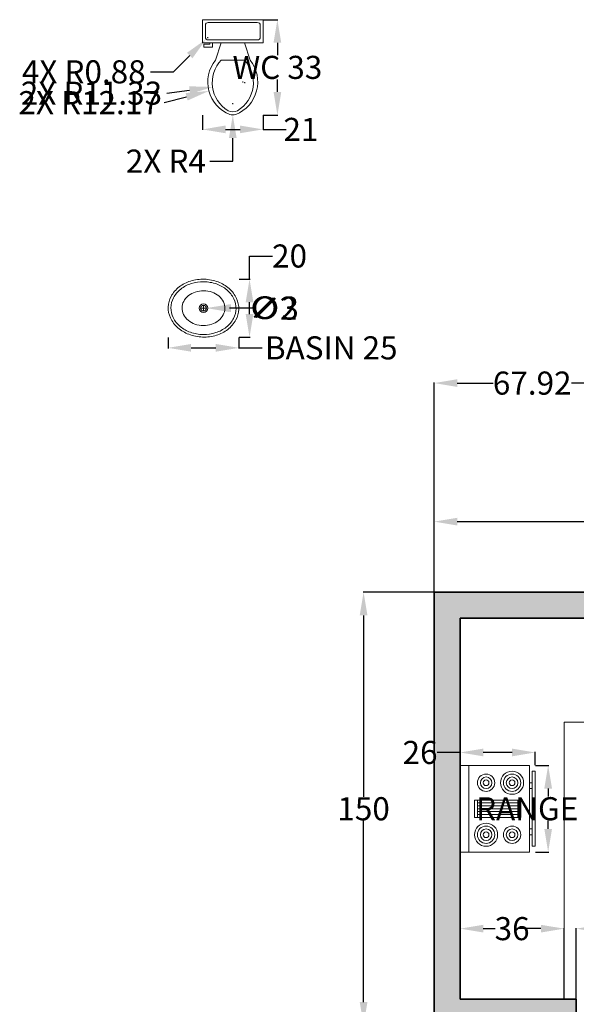
# Model space of a CAD drawing. Units: inches. Extents: x -52 to 678, y 23 to 685.
# Tile 6 of 11: x -52 to 141, y 334 to 675. Entities that reach past the tile are written whole.
import ezdxf

# ---------------------------------------------------------------- set-up
doc = ezdxf.new("R2010")
doc.units = ezdxf.units.IN
doc.header["$MEASUREMENT"] = 0
for name, color, linetype, lineweight in [('A-ANNO-DIMS', 2, 'Continuous', 18), ('A-EQPM', 8, 'Continuous', 18), ('A-FLOR-CASE', 8, 'Continuous', 18), ('A-FLOR-FIXT', 9, 'Continuous', 18), ('A-WALL', 7, 'Continuous', 35)]:
    doc.layers.add(name, color=color, linetype=linetype, lineweight=lineweight)
doc.layers.add('A-WALL-PATT', color=18, linetype='Continuous', lineweight=13, true_color=0x000000)
doc.styles.get("Standard").update_dxf_attribs({"font": 'arial.ttf'})
doc.dimstyles.get("Standard").update_dxf_attribs({"dimtxt": 8, "dimasz": 8, "dimexe": 0.18, "dimexo": 0.0625, "dimgap": 0.09, "dimtad": 0, "dimtih": 1, "dimtoh": 1, "dimdec": 0, "dimzin": 0, "dimdsep": 46, "dimlunit": 3, "dimtxsty": 'Standard', "dimcen": 0.09, "dimadec": 0, "dimazin": 0, "dimtfac": 1, "dimtdec": 0, "dimtofl": 0, "dimtmove": 0, "dimatfit": 3, "dimfxl": 1, "dimtolj": 1, "dimtzin": 0, "dimarcsym": 0})

# ---------------------------------------------------------------- blocks, each defined once
blk = doc.blocks.new('Range-Oven - 30 in top')
for p, q in [((0, -3), (30, -3)), ((12, -6), (18, -6)), ((13, -20), (13, -6)), ((14, -6), (14, -20)), ((15, -20), (15, -6)), ((16, -6), (16, -20)), ((17, -20), (17, -6)), ((18, -20), (12, -20)), ((6, -24), (6, -25)), ((8, -25), (8, -24)), ((22, -25), (22, -24)), ((24, -24), (24, -25))]:
    blk.add_line(p, q)
for points in [[(0, -24), (0, 0), (30, 0), (30, -24)], [(12, -21), (12, -5), (18, -5), (18, -21)], [(2, -26), (2, -25), (28, -25), (28, -26)]]:
    blk.add_lwpolyline(points, close=True)
for centre, radius in [((6, -9), 4), ((6, -9), 3), ((24, -9), 3), ((6, -9), 2), ((6, -9), 1), ((24, -9), 2), ((24, -9), 1), ((6, -18), 3), ((6, -18), 2), ((6, -18), 1), ((24, -18), 4), ((24, -18), 3), ((24, -18), 2), ((24, -18), 1)]:
    blk.add_circle(centre, radius)
blk = doc.blocks.new('Toilet - top')
for p, q in [((9.5, -6), (9.5, -2)), ((-10, -8.5), (-8, -8.5)), ((-10, -9.5), (-10, -8.5)), ((-7, -9.5), (-10, -9.5)), ((-8, -8.5), (-8, -8)), ((-7, -8), (-7, -9.5)), ((-4, -8), (-6, -14)), ((4, -8), (6, -14)), ((4, -14), (-4, -14))]:
    blk.add_line(p, q)
blk.add_lwpolyline([(10.5, -8), (10.5, 0), (-10.5, 0), (-10.5, -8)], close=True)
for points in [[(-9.5, -2), (-9.5, -6)], [(8.5, -1), (-8.5, -1)], [(-8.5, -7), (8.5, -7)]]:
    blk.add_lwpolyline(points)
for centre, radius, start, end in [((-8.62, -1.88), 0.884, 81.8699, 188.1301), ((8.62, -1.88), 0.884, 351.8699, 98.1301), ((-8.62, -6.12), 0.884, 171.8699, 278.1301), ((8.62, -6.12), 0.884, 261.8699, 8.1301), ((3.52, -21.58), 12.17, 141.4691, 247.9714), ((4.2, -21.82), 11.33, 136.3677, 238.9468), ((-3.52, -21.58), 12.17, 292.0284, 38.5307), ((-4.2, -21.82), 11.33, 301.053, 43.6321), ((0, -27.88), 4, 245.7318, 294.2682), ((0, -29), 4, 254.8605, 285.1395)]:
    blk.add_arc(centre, radius, start, end)
blk = doc.blocks.new('Sink - Oval top')
for p, q in [((-1, 0), (1, 0)), ((0, 1), (0, -1))]:
    blk.add_line(p, q)
for points in [[(-12.23, 0.39, 0.117634), (-11.46, -3.36, 0.104469), (-8.88, -6.8, 0.090016), (-5.08, -9.07, 0.08192), (-0.32, -10.02, 0.08192), (4.49, -9.38, 0.090016), (8.42, -7.36, 0.104469), (11.22, -4.09, 0.117634), (12.23, -0.39, 0.117634), (11.46, 3.36, 0.104469), (8.88, 6.8, 0.090016), (5.08, 9.07, 0.08192), (0.32, 10.02, 0.08192), (-4.49, 9.38, 0.090016), (-8.42, 7.36, 0.104469), (-11.22, 4.09, 0.117634)], [(-11.29, 0.16, 0.118622), (-10.52, -3.25, 0.104678), (-8.07, -6.36, 0.089562), (-4.54, -8.37, 0.081185), (-0.13, -9.15, 0.081185), (4.3, -8.49, 0.089562), (7.89, -6.58, 0.104678), (10.42, -3.55, 0.118622), (11.29, -0.16, 0.118622), (10.52, 3.25, 0.104678), (8.07, 6.36, 0.089562), (4.54, 8.37, 0.081185), (0.13, 9.15, 0.081185), (-4.3, 8.49, 0.089562), (-7.89, 6.58, 0.104678), (-10.42, 3.55, 0.118622)], [(-7.42, 0.08, 0.118283), (-6.91, -2.17, 0.104607), (-5.29, -4.21, 0.089718), (-2.97, -5.53, 0.081436), (-0.07, -6.04, 0.081436), (2.84, -5.59, 0.089718), (5.2, -4.33, 0.104607), (6.86, -2.32, 0.118283), (7.42, -0.08, 0.118283), (6.91, 2.17, 0.104607), (5.29, 4.21, 0.089718), (2.97, 5.53, 0.081436), (0.07, 6.04, 0.081436), (-2.84, 5.59, 0.089718), (-5.2, 4.33, 0.104607), (-6.86, 2.32, 0.118283)]]:
    blk.add_lwpolyline(points, format="xyb", close=True)
for radius in [1.5, 1]:
    blk.add_circle((0, 0), radius)
blk = doc.blocks.new('*D31')
at = {"layer": 'A-ANNO-DIMS', "color": 0, "lineweight": -2, "transparency": 16777216}
for p, q in [((126.67, 417.13), (131.29, 417.13)), ((131.11, 409.13), (131.11, 406.36)), ((131.11, 395.13), (131.11, 397.9)), ((126.67, 387.13), (131.29, 387.13))]:
    blk.add_line(p, q, dxfattribs=at)
at = {"layer": 'A-ANNO-DIMS', "color": 0, "transparency": 16777216}
for points in [[(129.77, 409.13), (132.44, 409.13), (131.11, 417.13)], [(129.77, 395.13), (132.44, 395.13), (131.11, 387.13)]]:
    blk.add_solid(points, dxfattribs=at)
at = {"layer": 'Defpoints', "color": 0, "transparency": 16777216}
for p in [(126.61, 417.13), (131.11, 417.13), (126.61, 387.13)]:
    blk.add_point(p, dxfattribs=at)
at = {"layer": 'A-ANNO-DIMS', "color": 0, "transparency": 16777216, "insert": (131.11, 402.13), "char_height": 8, "attachment_point": 5}
blk.add_mtext('\\A1;RANGE 30', dxfattribs=at)
blk = doc.blocks.new('*D32')
at = {"layer": 'A-ANNO-DIMS', "color": 0, "lineweight": -2, "transparency": 16777216}
for p, q in [((100.61, 421.63), (92.61, 421.63)), ((100.61, 417.19), (100.61, 421.81)), ((118.61, 421.63), (108.61, 421.63)), ((126.61, 417.19), (126.61, 421.81))]:
    blk.add_line(p, q, dxfattribs=at)
at = {"layer": 'A-ANNO-DIMS', "color": 0, "transparency": 16777216}
for points in [[(108.61, 422.96), (108.61, 420.29), (100.61, 421.63)], [(118.61, 422.96), (118.61, 420.29), (126.61, 421.63)]]:
    blk.add_solid(points, dxfattribs=at)
at = {"layer": 'Defpoints', "color": 0, "transparency": 16777216}
for p in [(100.61, 421.63), (100.61, 417.13), (126.61, 417.13)]:
    blk.add_point(p, dxfattribs=at)
at = {"layer": 'A-ANNO-DIMS', "color": 0, "transparency": 16777216, "insert": (86.72, 421.63), "char_height": 8, "attachment_point": 5}
blk.add_mtext('\\A1;26', dxfattribs=at)
blk = doc.blocks.new('*D33')
at = {"layer": 'A-ANNO-DIMS', "color": 0, "lineweight": -2, "transparency": 16777216}
for p, q in [((32.39, 675.49), (37.47, 675.49)), ((37.29, 667.49), (37.29, 663.19)), ((37.29, 650.44), (37.29, 654.73)), ((32.39, 642.44), (37.47, 642.44))]:
    blk.add_line(p, q, dxfattribs=at)
at = {"layer": 'A-ANNO-DIMS', "color": 0, "transparency": 16777216}
for points in [[(35.95, 667.49), (38.62, 667.49), (37.29, 675.49)], [(35.95, 650.44), (38.62, 650.44), (37.29, 642.44)]]:
    blk.add_solid(points, dxfattribs=at)
at = {"layer": 'Defpoints', "color": 0, "transparency": 16777216}
for p in [(32.33, 675.49), (37.29, 675.49), (32.33, 642.44)]:
    blk.add_point(p, dxfattribs=at)
at = {"layer": 'A-ANNO-DIMS', "color": 0, "transparency": 16777216, "insert": (37.29, 658.96), "char_height": 8, "attachment_point": 5}
blk.add_mtext('\\A1;WC 33', dxfattribs=at)
blk = doc.blocks.new('*D34')
at = {"layer": 'A-ANNO-DIMS', "color": 0, "lineweight": -2, "transparency": 16777216}
for p, q in [((11.33, 642.38), (11.33, 637.3)), ((32.33, 642.38), (32.33, 637.3)), ((19.33, 637.48), (24.33, 637.48)), ((32.33, 637.48), (40.33, 637.48))]:
    blk.add_line(p, q, dxfattribs=at)
at = {"layer": 'A-ANNO-DIMS', "color": 0, "transparency": 16777216}
for points in [[(19.33, 638.82), (19.33, 636.15), (11.33, 637.48)], [(24.33, 638.82), (24.33, 636.15), (32.33, 637.48)]]:
    blk.add_solid(points, dxfattribs=at)
at = {"layer": 'Defpoints', "color": 0, "transparency": 16777216}
for p in [(11.33, 642.44), (32.33, 642.44), (32.33, 637.48)]:
    blk.add_point(p, dxfattribs=at)
at = {"layer": 'A-ANNO-DIMS', "color": 0, "transparency": 16777216, "insert": (45.45, 637.48), "char_height": 8, "attachment_point": 5}
blk.add_mtext('\\A1;21', dxfattribs=at)
blk = doc.blocks.new('*D37')
at = {"layer": 'A-ANNO-DIMS', "color": 0, "lineweight": -2, "transparency": 16777216}
for p, q in [((-0.6, 565.42), (-0.6, 561.62)), ((23.95, 565.42), (23.95, 561.62)), ((7.4, 561.8), (15.95, 561.8)), ((23.95, 561.8), (31.95, 561.8))]:
    blk.add_line(p, q, dxfattribs=at)
at = {"layer": 'A-ANNO-DIMS', "color": 0, "transparency": 16777216}
for points in [[(7.4, 563.14), (7.4, 560.47), (-0.6, 561.8)], [(15.95, 563.14), (15.95, 560.47), (23.95, 561.8)]]:
    blk.add_solid(points, dxfattribs=at)
at = {"layer": 'Defpoints', "color": 0, "transparency": 16777216}
for p in [(-0.6, 565.49), (23.95, 565.49), (23.95, 561.8)]:
    blk.add_point(p, dxfattribs=at)
at = {"layer": 'A-ANNO-DIMS', "color": 0, "transparency": 16777216, "insert": (55.94, 561.8), "char_height": 8, "attachment_point": 5}
blk.add_mtext('\\A1;BASIN 25', dxfattribs=at)
blk = doc.blocks.new('*D38')
at = {"layer": 'A-ANNO-DIMS', "color": 0, "lineweight": -2, "transparency": 16777216}
for p, q in [((27.63, 585.62), (27.63, 593.62)), ((27.63, 593.62), (35.63, 593.62)), ((24.01, 585.62), (27.81, 585.62)), ((27.63, 573.49), (27.63, 577.62)), ((24.01, 565.49), (27.81, 565.49))]:
    blk.add_line(p, q, dxfattribs=at)
at = {"layer": 'A-ANNO-DIMS', "color": 0, "transparency": 16777216}
for points in [[(26.3, 577.62), (28.96, 577.62), (27.63, 585.62)], [(26.3, 573.49), (28.96, 573.49), (27.63, 565.49)]]:
    blk.add_solid(points, dxfattribs=at)
at = {"layer": 'Defpoints', "color": 0, "transparency": 16777216}
for p in [(23.95, 585.62), (27.63, 585.62), (23.95, 565.49)]:
    blk.add_point(p, dxfattribs=at)
at = {"layer": 'A-ANNO-DIMS', "color": 0, "transparency": 16777216, "insert": (41.5, 593.62), "char_height": 8, "attachment_point": 5}
blk.add_mtext('\\A1;20', dxfattribs=at)
blk = doc.blocks.new('*D41')
at = {"layer": 'A-ANNO-DIMS', "color": 0, "lineweight": -2, "transparency": 16777216}
for p, q in [((91.61, 477.19), (91.61, 501.77)), ((99.61, 501.59), (165.52, 501.59)), ((248.61, 501.59), (182.69, 501.59)), ((256.61, 477.19), (256.61, 501.77))]:
    blk.add_line(p, q, dxfattribs=at)
at = {"layer": 'A-ANNO-DIMS', "color": 0, "transparency": 16777216}
for points in [[(99.61, 502.92), (99.61, 500.25), (91.61, 501.59)], [(248.61, 502.92), (248.61, 500.25), (256.61, 501.59)]]:
    blk.add_solid(points, dxfattribs=at)
at = {"layer": 'Defpoints', "color": 0, "transparency": 16777216}
for p in [(256.61, 501.59), (91.61, 477.13), (256.61, 477.13)]:
    blk.add_point(p, dxfattribs=at)
at = {"layer": 'A-ANNO-DIMS', "color": 0, "transparency": 16777216, "insert": (174.11, 501.59), "char_height": 8, "attachment_point": 5}
blk.add_mtext('\\A1;165', dxfattribs=at)
blk = doc.blocks.new('*D45')
at = {"layer": 'A-ANNO-DIMS', "color": 0, "lineweight": -2, "transparency": 16777216}
for p, q in [((91.54, 477.13), (66.97, 477.13)), ((67.15, 469.13), (67.15, 406.3)), ((67.15, 335.13), (67.15, 397.95)), ((91.54, 327.13), (66.97, 327.13))]:
    blk.add_line(p, q, dxfattribs=at)
at = {"layer": 'A-ANNO-DIMS', "color": 0, "transparency": 16777216}
for points in [[(65.81, 469.13), (68.48, 469.13), (67.15, 477.13)], [(65.81, 335.13), (68.48, 335.13), (67.15, 327.13)]]:
    blk.add_solid(points, dxfattribs=at)
at = {"layer": 'Defpoints', "color": 0, "transparency": 16777216}
for p in [(67.15, 477.13), (91.61, 477.13), (91.61, 327.13)]:
    blk.add_point(p, dxfattribs=at)
at = {"layer": 'A-ANNO-DIMS', "color": 0, "transparency": 16777216, "insert": (67.15, 402.13), "char_height": 8, "attachment_point": 5}
blk.add_mtext('\\A1;150', dxfattribs=at)
blk = doc.blocks.new('*D63')
at = {"layer": 'A-ANNO-DIMS', "color": 0, "lineweight": -2, "transparency": 16777216}
for p, q in [((91.61, 477.19), (91.61, 549.77)), ((99.61, 549.59), (112, 549.59)), ((151.53, 549.59), (139.14, 549.59)), ((159.53, 477.19), (159.53, 549.77))]:
    blk.add_line(p, q, dxfattribs=at)
at = {"layer": 'A-ANNO-DIMS', "color": 0, "transparency": 16777216}
for points in [[(99.61, 550.92), (99.61, 548.25), (91.61, 549.59)], [(151.53, 550.92), (151.53, 548.25), (159.53, 549.59)]]:
    blk.add_solid(points, dxfattribs=at)
at = {"layer": 'Defpoints', "color": 0, "transparency": 16777216}
for p in [(159.53, 549.59), (91.61, 477.13), (159.53, 477.13)]:
    blk.add_point(p, dxfattribs=at)
at = {"layer": 'A-ANNO-DIMS', "color": 0, "transparency": 16777216, "insert": (125.57, 549.59), "char_height": 8, "attachment_point": 5}
blk.add_mtext('\\A1;67.92', dxfattribs=at)
blk = doc.blocks.new('*D71')
at = {"layer": 'A-ANNO-DIMS', "color": 0, "lineweight": -2, "transparency": 16777216}
for p, q in [((100.61, 336.19), (100.61, 360.77)), ((108.61, 360.59), (112.79, 360.59)), ((128.61, 360.59), (124.42, 360.59)), ((136.61, 336.19), (136.61, 360.77))]:
    blk.add_line(p, q, dxfattribs=at)
at = {"layer": 'A-ANNO-DIMS', "color": 0, "transparency": 16777216}
for points in [[(108.61, 361.92), (108.61, 359.25), (100.61, 360.59)], [(128.61, 361.92), (128.61, 359.25), (136.61, 360.59)]]:
    blk.add_solid(points, dxfattribs=at)
at = {"layer": 'Defpoints', "color": 0, "transparency": 16777216}
for p in [(136.61, 360.59), (100.61, 336.13), (136.61, 336.13)]:
    blk.add_point(p, dxfattribs=at)
at = {"layer": 'A-ANNO-DIMS', "color": 0, "transparency": 16777216, "insert": (118.61, 360.59), "char_height": 8, "attachment_point": 5}
blk.add_mtext('\\A1;36', dxfattribs=at)
blk = doc.blocks.new('*D72')
at = {"layer": 'A-ANNO-DIMS', "color": 0, "lineweight": -2, "transparency": 16777216}
for p, q in [((128.61, 360.59), (120.61, 360.59)), ((136.61, 336.19), (136.61, 360.77)), ((140.86, 336.19), (140.86, 360.77)), ((148.86, 360.59), (156.86, 360.59))]:
    blk.add_line(p, q, dxfattribs=at)
at = {"layer": 'A-ANNO-DIMS', "color": 0, "transparency": 16777216}
for points in [[(128.61, 361.92), (128.61, 359.25), (136.61, 360.59)], [(148.86, 361.92), (148.86, 359.25), (140.86, 360.59)]]:
    blk.add_solid(points, dxfattribs=at)
at = {"layer": 'Defpoints', "color": 0, "transparency": 16777216}
for p in [(140.86, 360.59), (136.61, 336.13), (140.86, 336.13)]:
    blk.add_point(p, dxfattribs=at)
at = {"layer": 'A-ANNO-DIMS', "color": 0, "transparency": 16777216, "insert": (170.62, 360.59), "char_height": 8, "attachment_point": 5}
blk.add_mtext('\\A1;4.259', dxfattribs=at)
blk = doc.blocks.new('*D105')
at = {"layer": 'A-ANNO-DIMS', "color": 0, "lineweight": -2, "transparency": 16777216}
for p, q in [((25.26, 653.91), (25.44, 653.91)), ((25.35, 653.82), (25.35, 654)), ((-1.9, 646.75), (5.84, 648.78))]:
    blk.add_line(p, q, dxfattribs=at)
at = {"layer": 'A-ANNO-DIMS', "color": 0, "transparency": 16777216}
blk.add_solid([(5.5, 650.07), (6.18, 647.49), (13.58, 650.81)], dxfattribs=at)
at = {"layer": 'Defpoints', "color": 0, "transparency": 16777216}
for p in [(25.35, 653.91), (13.58, 650.81)]:
    blk.add_point(p, dxfattribs=at)
at = {"layer": 'A-ANNO-DIMS', "color": 0, "transparency": 16777216, "insert": (-27.97, 646.75), "char_height": 8, "attachment_point": 5}
blk.add_mtext('\\A1;2X R12.17', dxfattribs=at)
blk = doc.blocks.new('*D106')
at = {"layer": 'A-ANNO-DIMS', "color": 0, "lineweight": -2, "transparency": 16777216}
for p, q in [((25.94, 653.67), (26.12, 653.67)), ((26.03, 653.58), (26.03, 653.76)), ((-1.06, 650.03), (6.87, 651.09))]:
    blk.add_line(p, q, dxfattribs=at)
at = {"layer": 'A-ANNO-DIMS', "color": 0, "transparency": 16777216}
blk.add_solid([(6.69, 652.42), (7.05, 649.77), (14.8, 652.16)], dxfattribs=at)
at = {"layer": 'Defpoints', "color": 0, "transparency": 16777216}
for p in [(14.8, 652.16), (26.03, 653.67)]:
    blk.add_point(p, dxfattribs=at)
at = {"layer": 'A-ANNO-DIMS', "color": 0, "transparency": 16777216, "insert": (-27.14, 650.03), "char_height": 8, "attachment_point": 5}
blk.add_mtext('\\A1;2X R11.33', dxfattribs=at)
blk = doc.blocks.new('*D107')
at = {"layer": 'A-ANNO-DIMS', "color": 0, "lineweight": -2, "transparency": 16777216}
for p, q in [((21.74, 646.49), (21.92, 646.49)), ((21.83, 646.4), (21.83, 646.58)), ((21.83, 626.49), (21.83, 634.49)), ((13.83, 626.49), (21.83, 626.49))]:
    blk.add_line(p, q, dxfattribs=at)
at = {"layer": 'A-ANNO-DIMS', "color": 0, "transparency": 16777216}
blk.add_solid([(20.49, 634.49), (23.16, 634.49), (21.83, 642.49)], dxfattribs=at)
at = {"layer": 'Defpoints', "color": 0, "transparency": 16777216}
for p in [(21.83, 646.49), (21.83, 642.49)]:
    blk.add_point(p, dxfattribs=at)
at = {"layer": 'A-ANNO-DIMS', "color": 0, "transparency": 16777216, "insert": (-1.36, 626.49), "char_height": 8, "attachment_point": 5}
blk.add_mtext('\\A1;2X R4', dxfattribs=at)
blk = doc.blocks.new('*D108')
at = {"layer": 'A-ANNO-DIMS', "color": 0, "lineweight": -2, "transparency": 16777216}
for p, q in [((13.11, 669.36), (13.29, 669.36)), ((13.2, 669.27), (13.2, 669.45)), ((1.26, 657.43), (6.92, 663.08)), ((-6.74, 657.43), (1.26, 657.43))]:
    blk.add_line(p, q, dxfattribs=at)
at = {"layer": 'A-ANNO-DIMS', "color": 0, "transparency": 16777216}
blk.add_solid([(5.98, 664.03), (7.86, 662.14), (12.58, 668.74)], dxfattribs=at)
at = {"layer": 'Defpoints', "color": 0, "transparency": 16777216}
for p in [(12.58, 668.74), (13.2, 669.36)]:
    blk.add_point(p, dxfattribs=at)
at = {"layer": 'A-ANNO-DIMS', "color": 0, "transparency": 16777216, "insert": (-29.81, 657.43), "char_height": 8, "attachment_point": 5}
blk.add_mtext('\\A1;4X R0.88', dxfattribs=at)
blk = doc.blocks.new('*D109')
at = {"layer": 'A-ANNO-DIMS', "color": 0, "lineweight": -2, "transparency": 16777216}
for p, q in [((11.58, 575.56), (11.76, 575.56)), ((11.67, 575.47), (11.67, 575.65)), ((29.17, 575.56), (21.17, 575.56))]:
    blk.add_line(p, q, dxfattribs=at)
at = {"layer": 'A-ANNO-DIMS', "color": 0, "transparency": 16777216}
blk.add_solid([(21.17, 576.89), (21.17, 574.22), (13.17, 575.56)], dxfattribs=at)
at = {"layer": 'Defpoints', "color": 0, "transparency": 16777216}
for p in [(10.17, 575.56), (13.17, 575.56)]:
    blk.add_point(p, dxfattribs=at)
at = {"layer": 'A-ANNO-DIMS', "color": 0, "transparency": 16777216, "insert": (36.24, 575.56), "char_height": 8, "attachment_point": 5}
blk.add_mtext('\\A1;∅3', dxfattribs=at)
blk = doc.blocks.new('*D110')
at = {"layer": 'A-ANNO-DIMS', "color": 0, "lineweight": -2, "transparency": 16777216}
for p, q in [((11.58, 575.56), (11.76, 575.56)), ((11.67, 575.47), (11.67, 575.65)), ((28.67, 575.56), (20.67, 575.56))]:
    blk.add_line(p, q, dxfattribs=at)
at = {"layer": 'A-ANNO-DIMS', "color": 0, "transparency": 16777216}
blk.add_solid([(20.67, 576.89), (20.67, 574.22), (12.67, 575.56)], dxfattribs=at)
at = {"layer": 'Defpoints', "color": 0, "transparency": 16777216}
for p in [(10.67, 575.56), (12.67, 575.56)]:
    blk.add_point(p, dxfattribs=at)
at = {"layer": 'A-ANNO-DIMS', "color": 0, "transparency": 16777216, "insert": (35.69, 575.56), "char_height": 8, "attachment_point": 5}
blk.add_mtext('\\A1;∅2', dxfattribs=at)

msp = doc.modelspace()

# ---------------------------------------------------------------- hatches: boundary and pattern name
at = {"layer": 'A-WALL-PATT'}
h = msp.add_hatch(color=256, dxfattribs=at)
h.dxf.hatch_style = 1
h.paths.add_polyline_path([(100.6053, 336.1267), (100.6053, 468.1267), (159.5302, 468.1267), (159.5302, 477.1267), (91.6053, 477.1267), (91.6053, 327.1267), (140.8548, 327.1267), (140.8548, 336.1267), (137.7032, 336.1267)])

# ---------------------------------------------------------------- linework, layer by layer
at = {"layer": 'A-FLOR-CASE'}
for p, q in [((218.4552, 432.1267), (136.6053, 432.1267)), ((136.6053, 336.1267), (136.6053, 432.1267)), ((100.6053, 336.1267), (136.6053, 336.1267))]:
    msp.add_line(p, q, dxfattribs=at)
at = {"layer": 'A-WALL'}
for p, q in [((91.6053, 477.1267), (91.6053, 327.1267)), ((91.6053, 477.1267), (159.5302, 477.1267)), ((100.6053, 468.1267), (100.6053, 336.1267)), ((100.6053, 468.1267), (159.5302, 468.1267)), ((100.6053, 336.1267), (137.7032, 336.1267)), ((137.7032, 336.1267), (140.8548, 336.1267)), ((140.8548, 336.1267), (140.8548, 327.1267))]:
    msp.add_line(p, q, dxfattribs=at)

# ---------------------------------------------------------------- block references
at = {"layer": 'A-EQPM', "rotation": 90}
msp.add_blockref('Range-Oven - 30 in top', (100.6053, 387.1267), dxfattribs=at)
at = {"layer": 'A-FLOR-FIXT'}
for name, p in [('Toilet - top', (21.8294, 675.4867)), ('Sink - Oval top', (11.6716, 575.5557))]:
    msp.add_blockref(name, p, dxfattribs=at)

# ---------------------------------------------------------------- dimensions: what is measured, and where the dimension line sits
at = {"layer": 'A-ANNO-DIMS'}
for base, p1, p2, text, picture, middle in [((37.2863, 675.4867), (32.3294, 642.4405), (32.3294, 675.4867), 'WC <>', '*D33', (37.2863, 658.9636)), ((131.1053, 417.1267), (126.6053, 387.1267), (126.6053, 417.1267), 'RANGE <>', '*D31', (131.1053, 402.1267))]:
    dim = msp.add_linear_dim(base=base, p1=p1, p2=p2, angle=90, text=text, dimstyle='Standard', override={"dimdec": 0, "dimlfac": 1, "dimrnd": 0, "dimzin": 0, "dimdsep": 46, "dimlunit": 2}, dxfattribs=at)
    dim.commit()
    dim.dimension.update_dxf_attribs({"geometry": picture, "text_midpoint": middle})
for center, mpoint, text, override, picture, middle in [((13.2044, 669.3617), (12.579, 668.737), '4X <>', {"dimdec": 2, "dimlfac": 1, "dimrnd": 0, "dimzin": 0, "dimdsep": 46, "dimlunit": 2}, '*D108', (-29.8133, 657.4297)), ((26.0294, 653.6693), (14.8012, 652.16), '2X <>', {"dimdec": 2, "dimlfac": 1, "dimrnd": 0, "dimzin": 0, "dimdsep": 46, "dimlunit": 2}, '*D106', (-27.1353, 650.0285)), ((25.349, 653.9062), (13.5793, 650.8141), '2X <>', {"dimdec": 2, "dimlfac": 1, "dimrnd": 0, "dimzin": 0, "dimdsep": 46, "dimlunit": 2}, '*D105', (-27.9746, 646.7485)), ((21.8294, 646.4867), (21.829, 642.4867), '2X <>', {"dimdec": 0, "dimlfac": 1, "dimrnd": 0, "dimzin": 0, "dimdsep": 46, "dimlunit": 2}, '*D107', (-1.3596, 626.4867))]:
    dim = msp.add_radius_dim(center=center, mpoint=mpoint, text=text, dimstyle='Standard', override=override, dxfattribs=at)
    dim.commit()
    dim.dimension.update_dxf_attribs({"geometry": picture, "text_midpoint": middle})
for base, p1, p2, override, picture, middle in [((32.3294, 637.4835), (11.3294, 642.4405), (32.3294, 642.4405), {"dimdec": 0, "dimlfac": 1, "dimrnd": 0, "dimzin": 0, "dimdsep": 46, "dimlunit": 2}, '*D34', (45.4453, 637.4835)), ((159.5302, 549.5867), (91.6053, 477.1267), (159.5302, 477.1267), {"dimdec": 2, "dimlfac": 1, "dimrnd": 0, "dimzin": 0, "dimdsep": 46, "dimlunit": 2}, '*D63', (125.5677, 549.5867)), ((136.6053, 360.5867), (100.6053, 336.1267), (136.6053, 336.1267), {"dimdec": 0, "dimlfac": 1, "dimrnd": 0, "dimzin": 0, "dimdsep": 46, "dimlunit": 2}, '*D71', (118.6053, 360.5867))]:
    dim = msp.add_linear_dim(base=base, p1=p1, p2=p2, dimstyle='Standard', override=override, dxfattribs=at)
    dim.commit()
    dim.dimension.update_dxf_attribs({"geometry": picture, "text_midpoint": middle})
for base, p1, p2, angle, override, picture, middle in [((27.6297, 585.624), (23.947, 565.4874), (23.947, 585.624), 90, {"dimdec": 0, "dimlfac": 1, "dimrnd": 0, "dimzin": 0, "dimdsep": 46, "dimlunit": 2}, '*D38', (41.5041, 593.624)), ((256.6053, 501.5867), (91.6053, 477.1267), (256.6053, 477.1267), 0, {"dimdec": 0, "dimlfac": 1, "dimrnd": 0, "dimzin": 0, "dimdsep": 46, "dimlunit": 2}, '*D41', (174.1053, 501.5867)), ((67.1453, 477.1267), (91.6053, 327.1267), (91.6053, 477.1267), 90, {"dimdec": 0, "dimlfac": 1, "dimrnd": 0, "dimzin": 0, "dimdsep": 46, "dimlunit": 2}, '*D45', (67.1453, 402.1267)), ((100.6053, 421.6267), (126.6053, 417.1267), (100.6053, 417.1267), 180, {"dimdec": 0, "dimlfac": 1, "dimrnd": 0, "dimzin": 0, "dimdsep": 46, "dimlunit": 2}, '*D32', (86.7199, 421.6267)), ((140.8647, 360.5867), (136.6053, 336.1267), (140.8646, 336.1267), 359.999705, {"dimdec": 3, "dimlfac": 1, "dimrnd": 0, "dimzin": 0, "dimdsep": 46, "dimlunit": 2}, '*D72', (170.6219, 360.5866))]:
    dim = msp.add_linear_dim(base=base, p1=p1, p2=p2, angle=angle, dimstyle='Standard', override=override, dxfattribs=at)
    dim.commit()
    dim.dimension.update_dxf_attribs({"geometry": picture, "text_midpoint": middle})
dim = msp.add_diameter_dim_2p(p1=(10.1716, 575.5555), p2=(13.1716, 575.556), dimstyle='Standard', override={"dimdec": 0, "dimlfac": 1, "dimrnd": 0, "dimzin": 0, "dimdsep": 46, "dimlunit": 2}, dxfattribs=at)
dim.commit()
dim.dimension.update_dxf_attribs({"geometry": '*D109', "text_midpoint": (29.1716, 575.5588), "dimtype": 163})
dim = msp.add_diameter_dim_2p(p1=(10.6716, 575.5555), p2=(12.6716, 575.556), dimstyle='Standard', override={"dimdec": 0, "dimlfac": 1, "dimrnd": 0, "dimzin": 0, "dimdsep": 46, "dimlunit": 2}, dxfattribs=at)
dim.commit()
dim.dimension.update_dxf_attribs({"geometry": '*D110', "text_midpoint": (28.6716, 575.5602)})
dim = msp.add_linear_dim(base=(23.947, 561.8048), p1=(-0.6039, 565.4874), p2=(23.947, 565.4874), text='BASIN <>', dimstyle='Standard', override={"dimdec": 0, "dimlfac": 1, "dimrnd": 0, "dimzin": 0, "dimdsep": 46, "dimlunit": 2}, dxfattribs=at)
dim.commit()
dim.dimension.update_dxf_attribs({"geometry": '*D37', "text_midpoint": (55.9415, 561.8048)})

doc.saveas('drawing.dxf')
